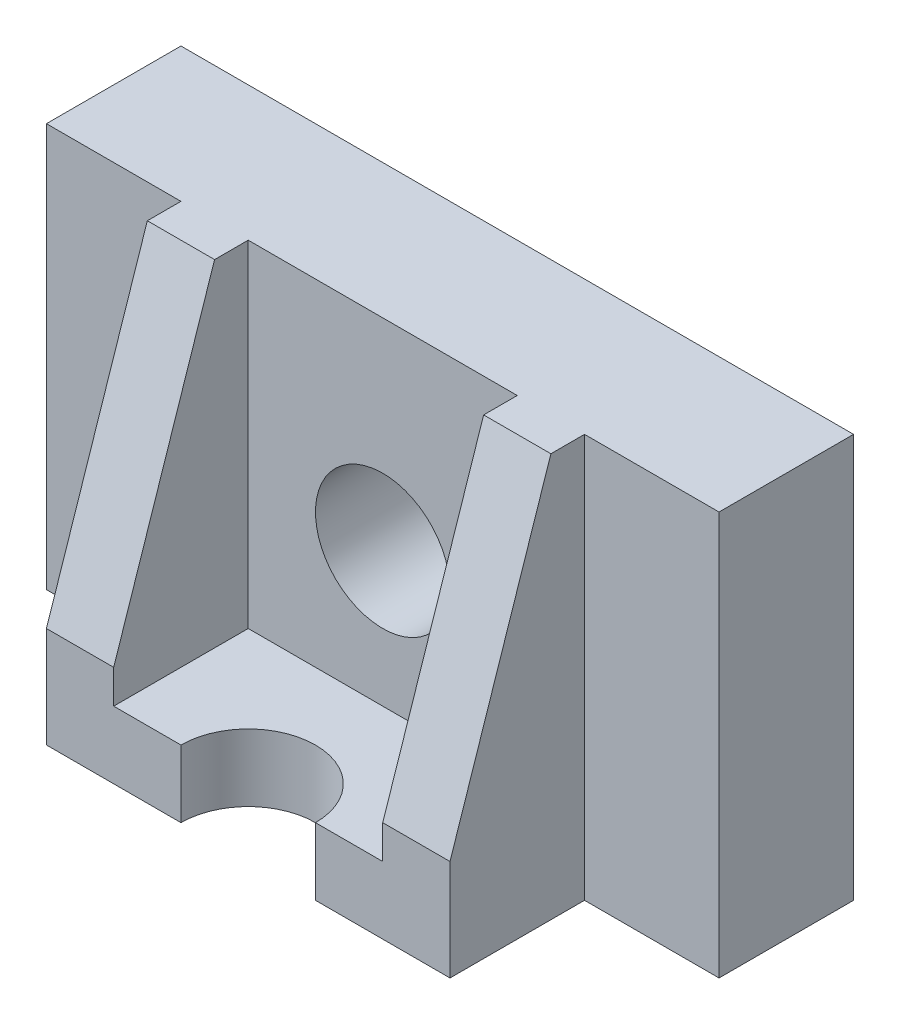
ISO-10303-21;
HEADER;
FILE_DESCRIPTION(('STEP AP214'),'2;1');
FILE_NAME('part.step','',(''),(''),'','','');
FILE_SCHEMA(('AUTOMOTIVE_DESIGN { 1 0 10303 214 1 1 1 1 }'));
ENDSEC;
DATA;
#1=APPLICATION_CONTEXT('core data for automotive mechanical design processes');
#2=APPLICATION_PROTOCOL_DEFINITION('international standard','automotive_design',2000,#1);
#3=PRODUCT_CONTEXT('',#1,'mechanical');
#4=PRODUCT('Part','Part','',(#3));
#5=PRODUCT_RELATED_PRODUCT_CATEGORY('part','',(#4));
#6=PRODUCT_DEFINITION_FORMATION('','',#4);
#7=PRODUCT_DEFINITION_CONTEXT('part definition',#1,'design');
#8=PRODUCT_DEFINITION('design','',#6,#7);
#9=PRODUCT_DEFINITION_SHAPE('','',#8);
#10=(LENGTH_UNIT() NAMED_UNIT(*) SI_UNIT(.MILLI.,.METRE.));
#11=(NAMED_UNIT(*) PLANE_ANGLE_UNIT() SI_UNIT($,.RADIAN.));
#12=(NAMED_UNIT(*) SI_UNIT($,.STERADIAN.) SOLID_ANGLE_UNIT());
#13=UNCERTAINTY_MEASURE_WITH_UNIT(LENGTH_MEASURE(1.E-05),#10,'distance_accuracy_value','');
#14=(GEOMETRIC_REPRESENTATION_CONTEXT(3) GLOBAL_UNCERTAINTY_ASSIGNED_CONTEXT((#13)) GLOBAL_UNIT_ASSIGNED_CONTEXT((#10,
#11,#12)) REPRESENTATION_CONTEXT('',''));
#15=CARTESIAN_POINT('',(0.,0.,0.));
#16=DIRECTION('',(0.,0.,1.));
#17=DIRECTION('',(1.,0.,0.));
#18=AXIS2_PLACEMENT_3D('',#15,#16,#17);
#19=CARTESIAN_POINT('',(0.,0.,20.));
#20=DIRECTION('',(0.,0.,1.));
#21=DIRECTION('',(1.,0.,0.));
#22=AXIS2_PLACEMENT_3D('',#19,#20,#21);
#23=PLANE('',#22);
#24=CARTESIAN_POINT('',(50.,30.,20.));
#25=DIRECTION('',(0.,0.,1.));
#26=DIRECTION('',(1.,0.,0.));
#27=AXIS2_PLACEMENT_3D('',#24,#25,#26);
#28=CIRCLE('',#27,10.);
#29=CARTESIAN_POINT('',(60.,30.,20.));
#30=VERTEX_POINT('',#29);
#31=EDGE_CURVE('E217',#30,#30,#28,.T.);
#32=ORIENTED_EDGE('',*,*,#31,.F.);
#33=EDGE_LOOP('',(#32));
#34=FACE_BOUND('',#33,.T.);
#35=DIRECTION('',(-1.,0.,0.));
#36=VECTOR('',#35,1.);
#37=CARTESIAN_POINT('',(100.,60.,20.));
#38=LINE('',#37,#36);
#39=CARTESIAN_POINT('',(70.,60.,20.));
#40=VERTEX_POINT('',#39);
#41=CARTESIAN_POINT('',(30.,60.,20.));
#42=VERTEX_POINT('',#41);
#43=EDGE_CURVE('E245',#40,#42,#38,.T.);
#44=ORIENTED_EDGE('',*,*,#43,.T.);
#45=DIRECTION('',(0.,-1.,0.));
#46=VECTOR('',#45,1.);
#47=CARTESIAN_POINT('',(30.,60.,20.));
#48=LINE('',#47,#46);
#49=CARTESIAN_POINT('',(30.,10.,20.));
#50=VERTEX_POINT('',#49);
#51=EDGE_CURVE('E274',#42,#50,#48,.T.);
#52=ORIENTED_EDGE('',*,*,#51,.T.);
#53=DIRECTION('',(1.,0.,0.));
#54=VECTOR('',#53,1.);
#55=CARTESIAN_POINT('',(20.,10.,20.));
#56=LINE('',#55,#54);
#57=CARTESIAN_POINT('',(70.,10.,20.));
#58=VERTEX_POINT('',#57);
#59=EDGE_CURVE('E186',#50,#58,#56,.T.);
#60=ORIENTED_EDGE('',*,*,#59,.T.);
#61=DIRECTION('',(0.,1.,0.));
#62=VECTOR('',#61,1.);
#63=CARTESIAN_POINT('',(70.,60.,20.));
#64=LINE('',#63,#62);
#65=EDGE_CURVE('E277',#58,#40,#64,.T.);
#66=ORIENTED_EDGE('',*,*,#65,.T.);
#67=EDGE_LOOP('',(#44,#52,#60,#66));
#68=FACE_BOUND('',#67,.T.);
#69=ADVANCED_FACE('F44',(#34,#68),#23,.T.);
#70=CARTESIAN_POINT('',(50.,10.,40.));
#71=DIRECTION('',(0.,-1.,0.));
#72=DIRECTION('',(0.,0.,-1.));
#73=AXIS2_PLACEMENT_3D('',#70,#71,#72);
#74=PLANE('',#73);
#75=DIRECTION('',(0.,0.,1.));
#76=VECTOR('',#75,1.);
#77=CARTESIAN_POINT('',(30.,10.,20.));
#78=LINE('',#77,#76);
#79=CARTESIAN_POINT('',(30.,10.,40.));
#80=VERTEX_POINT('',#79);
#81=EDGE_CURVE('E175',#50,#80,#78,.T.);
#82=ORIENTED_EDGE('',*,*,#81,.T.);
#83=DIRECTION('',(-1.,0.,0.));
#84=VECTOR('',#83,1.);
#85=CARTESIAN_POINT('',(20.,10.,40.));
#86=LINE('',#85,#84);
#87=CARTESIAN_POINT('',(40.,10.,40.));
#88=VERTEX_POINT('',#87);
#89=EDGE_CURVE('E187',#88,#80,#86,.T.);
#90=ORIENTED_EDGE('',*,*,#89,.F.);
#91=CARTESIAN_POINT('',(50.,10.,40.));
#92=DIRECTION('',(0.,1.,0.));
#93=DIRECTION('',(0.,0.,-1.));
#94=AXIS2_PLACEMENT_3D('',#91,#92,#93);
#95=CIRCLE('',#94,10.);
#96=CARTESIAN_POINT('',(60.,10.,40.));
#97=VERTEX_POINT('',#96);
#98=EDGE_CURVE('E196',#97,#88,#95,.T.);
#99=ORIENTED_EDGE('',*,*,#98,.F.);
#100=DIRECTION('',(-1.,0.,0.));
#101=VECTOR('',#100,1.);
#102=CARTESIAN_POINT('',(80.,10.,40.));
#103=LINE('',#102,#101);
#104=CARTESIAN_POINT('',(70.,10.,40.));
#105=VERTEX_POINT('',#104);
#106=EDGE_CURVE('E199',#105,#97,#103,.T.);
#107=ORIENTED_EDGE('',*,*,#106,.F.);
#108=DIRECTION('',(0.,0.,-1.));
#109=VECTOR('',#108,1.);
#110=CARTESIAN_POINT('',(70.,10.,20.));
#111=LINE('',#110,#109);
#112=EDGE_CURVE('E292',#105,#58,#111,.T.);
#113=ORIENTED_EDGE('',*,*,#112,.T.);
#114=ORIENTED_EDGE('',*,*,#59,.F.);
#115=EDGE_LOOP('',(#82,#90,#99,#107,#113,#114));
#116=FACE_BOUND('',#115,.T.);
#117=ADVANCED_FACE('F183',(#116),#74,.F.);
#118=CARTESIAN_POINT('',(100.,60.,20.));
#119=VERTEX_POINT('',#118);
#120=CARTESIAN_POINT('',(80.,60.,20.));
#121=VERTEX_POINT('',#120);
#122=EDGE_CURVE('E238',#119,#121,#38,.T.);
#123=ORIENTED_EDGE('',*,*,#122,.T.);
#124=DIRECTION('',(0.,-1.,0.));
#125=VECTOR('',#124,1.);
#126=CARTESIAN_POINT('',(80.,10.,20.));
#127=LINE('',#126,#125);
#128=CARTESIAN_POINT('',(80.,0.,20.));
#129=VERTEX_POINT('',#128);
#130=EDGE_CURVE('E193',#121,#129,#127,.T.);
#131=ORIENTED_EDGE('',*,*,#130,.T.);
#132=DIRECTION('',(1.,0.,0.));
#133=VECTOR('',#132,1.);
#134=CARTESIAN_POINT('',(0.,0.,20.));
#135=LINE('',#134,#133);
#136=CARTESIAN_POINT('',(100.,0.,20.));
#137=VERTEX_POINT('',#136);
#138=EDGE_CURVE('E234',#129,#137,#135,.T.);
#139=ORIENTED_EDGE('',*,*,#138,.T.);
#140=DIRECTION('',(0.,1.,0.));
#141=VECTOR('',#140,1.);
#142=CARTESIAN_POINT('',(100.,0.,20.));
#143=LINE('',#142,#141);
#144=EDGE_CURVE('E236',#137,#119,#143,.T.);
#145=ORIENTED_EDGE('',*,*,#144,.T.);
#146=EDGE_LOOP('',(#123,#131,#139,#145));
#147=FACE_BOUND('',#146,.T.);
#148=ADVANCED_FACE('F327',(#147),#23,.T.);
#149=CARTESIAN_POINT('',(0.,60.,20.));
#150=DIRECTION('',(1.,0.,0.));
#151=DIRECTION('',(0.,0.,-1.));
#152=AXIS2_PLACEMENT_3D('',#149,#150,#151);
#153=PLANE('',#152);
#154=DIRECTION('',(0.,-1.,0.));
#155=VECTOR('',#154,1.);
#156=CARTESIAN_POINT('',(0.,60.,0.));
#157=LINE('',#156,#155);
#158=CARTESIAN_POINT('',(0.,60.,0.));
#159=VERTEX_POINT('',#158);
#160=CARTESIAN_POINT('',(0.,0.,0.));
#161=VERTEX_POINT('',#160);
#162=EDGE_CURVE('E230',#159,#161,#157,.T.);
#163=ORIENTED_EDGE('',*,*,#162,.T.);
#164=DIRECTION('',(0.,0.,-1.));
#165=VECTOR('',#164,1.);
#166=CARTESIAN_POINT('',(0.,0.,20.));
#167=LINE('',#166,#165);
#168=CARTESIAN_POINT('',(0.,0.,20.));
#169=VERTEX_POINT('',#168);
#170=EDGE_CURVE('E11',#169,#161,#167,.T.);
#171=ORIENTED_EDGE('',*,*,#170,.F.);
#172=DIRECTION('',(0.,-1.,0.));
#173=VECTOR('',#172,1.);
#174=CARTESIAN_POINT('',(0.,60.,20.));
#175=LINE('',#174,#173);
#176=CARTESIAN_POINT('',(0.,60.,20.));
#177=VERTEX_POINT('',#176);
#178=EDGE_CURVE('E235',#177,#169,#175,.T.);
#179=ORIENTED_EDGE('',*,*,#178,.F.);
#180=DIRECTION('',(0.,0.,-1.));
#181=VECTOR('',#180,1.);
#182=CARTESIAN_POINT('',(0.,60.,20.));
#183=LINE('',#182,#181);
#184=EDGE_CURVE('E241',#177,#159,#183,.T.);
#185=ORIENTED_EDGE('',*,*,#184,.T.);
#186=EDGE_LOOP('',(#163,#171,#179,#185));
#187=FACE_BOUND('',#186,.T.);
#188=ADVANCED_FACE('F50',(#187),#153,.F.);
#189=CARTESIAN_POINT('',(0.,0.,20.));
#190=DIRECTION('',(0.,1.,0.));
#191=DIRECTION('',(0.,0.,1.));
#192=AXIS2_PLACEMENT_3D('',#189,#190,#191);
#193=PLANE('',#192);
#194=DIRECTION('',(1.,0.,0.));
#195=VECTOR('',#194,1.);
#196=CARTESIAN_POINT('',(0.,0.,0.));
#197=LINE('',#196,#195);
#198=CARTESIAN_POINT('',(100.,0.,0.));
#199=VERTEX_POINT('',#198);
#200=EDGE_CURVE('E244',#161,#199,#197,.T.);
#201=ORIENTED_EDGE('',*,*,#200,.T.);
#202=DIRECTION('',(0.,0.,-1.));
#203=VECTOR('',#202,1.);
#204=CARTESIAN_POINT('',(100.,0.,20.));
#205=LINE('',#204,#203);
#206=EDGE_CURVE('E52',#137,#199,#205,.T.);
#207=ORIENTED_EDGE('',*,*,#206,.F.);
#208=ORIENTED_EDGE('',*,*,#138,.F.);
#209=DIRECTION('',(0.,0.,1.));
#210=VECTOR('',#209,1.);
#211=CARTESIAN_POINT('',(80.,0.,20.));
#212=LINE('',#211,#210);
#213=CARTESIAN_POINT('',(80.,0.,40.));
#214=VERTEX_POINT('',#213);
#215=EDGE_CURVE('E58',#129,#214,#212,.T.);
#216=ORIENTED_EDGE('',*,*,#215,.T.);
#217=DIRECTION('',(-1.,0.,0.));
#218=VECTOR('',#217,1.);
#219=CARTESIAN_POINT('',(80.,0.,40.));
#220=LINE('',#219,#218);
#221=CARTESIAN_POINT('',(60.,0.,40.));
#222=VERTEX_POINT('',#221);
#223=EDGE_CURVE('E205',#214,#222,#220,.T.);
#224=ORIENTED_EDGE('',*,*,#223,.T.);
#225=CARTESIAN_POINT('',(50.,0.,40.));
#226=DIRECTION('',(0.,1.,0.));
#227=DIRECTION('',(0.,0.,-1.));
#228=AXIS2_PLACEMENT_3D('',#225,#226,#227);
#229=CIRCLE('',#228,10.);
#230=CARTESIAN_POINT('',(40.,0.,40.));
#231=VERTEX_POINT('',#230);
#232=EDGE_CURVE('E209',#222,#231,#229,.T.);
#233=ORIENTED_EDGE('',*,*,#232,.T.);
#234=DIRECTION('',(-1.,0.,0.));
#235=VECTOR('',#234,1.);
#236=CARTESIAN_POINT('',(20.,0.,40.));
#237=LINE('',#236,#235);
#238=CARTESIAN_POINT('',(20.,0.,40.));
#239=VERTEX_POINT('',#238);
#240=EDGE_CURVE('E215',#231,#239,#237,.T.);
#241=ORIENTED_EDGE('',*,*,#240,.T.);
#242=DIRECTION('',(0.,0.,-1.));
#243=VECTOR('',#242,1.);
#244=CARTESIAN_POINT('',(20.,0.,20.));
#245=LINE('',#244,#243);
#246=CARTESIAN_POINT('',(20.,0.,20.));
#247=VERTEX_POINT('',#246);
#248=EDGE_CURVE('E213',#239,#247,#245,.T.);
#249=ORIENTED_EDGE('',*,*,#248,.T.);
#250=EDGE_CURVE('E96',#169,#247,#135,.T.);
#251=ORIENTED_EDGE('',*,*,#250,.F.);
#252=ORIENTED_EDGE('',*,*,#170,.T.);
#253=EDGE_LOOP('',(#201,#207,#208,#216,#224,#233,#241,#249,#251,#252));
#254=FACE_BOUND('',#253,.T.);
#255=ADVANCED_FACE('F318',(#254),#193,.F.);
#256=CARTESIAN_POINT('',(100.,0.,20.));
#257=DIRECTION('',(-1.,0.,0.));
#258=DIRECTION('',(0.,0.,1.));
#259=AXIS2_PLACEMENT_3D('',#256,#257,#258);
#260=PLANE('',#259);
#261=DIRECTION('',(0.,1.,0.));
#262=VECTOR('',#261,1.);
#263=CARTESIAN_POINT('',(100.,0.,0.));
#264=LINE('',#263,#262);
#265=CARTESIAN_POINT('',(100.,60.,0.));
#266=VERTEX_POINT('',#265);
#267=EDGE_CURVE('E250',#199,#266,#264,.T.);
#268=ORIENTED_EDGE('',*,*,#267,.T.);
#269=DIRECTION('',(0.,0.,-1.));
#270=VECTOR('',#269,1.);
#271=CARTESIAN_POINT('',(100.,60.,20.));
#272=LINE('',#271,#270);
#273=EDGE_CURVE('E252',#119,#266,#272,.T.);
#274=ORIENTED_EDGE('',*,*,#273,.F.);
#275=ORIENTED_EDGE('',*,*,#144,.F.);
#276=ORIENTED_EDGE('',*,*,#206,.T.);
#277=EDGE_LOOP('',(#268,#274,#275,#276));
#278=FACE_BOUND('',#277,.T.);
#279=ADVANCED_FACE('F260',(#278),#260,.F.);
#280=CARTESIAN_POINT('',(100.,60.,20.));
#281=DIRECTION('',(0.,-1.,0.));
#282=DIRECTION('',(0.,0.,-1.));
#283=AXIS2_PLACEMENT_3D('',#280,#281,#282);
#284=PLANE('',#283);
#285=DIRECTION('',(-1.,0.,0.));
#286=VECTOR('',#285,1.);
#287=CARTESIAN_POINT('',(100.,60.,0.));
#288=LINE('',#287,#286);
#289=EDGE_CURVE('E91',#266,#159,#288,.T.);
#290=ORIENTED_EDGE('',*,*,#289,.T.);
#291=ORIENTED_EDGE('',*,*,#184,.F.);
#292=CARTESIAN_POINT('',(20.,60.,20.));
#293=VERTEX_POINT('',#292);
#294=EDGE_CURVE('E67',#293,#177,#38,.T.);
#295=ORIENTED_EDGE('',*,*,#294,.F.);
#296=DIRECTION('',(0.,0.,-1.));
#297=VECTOR('',#296,1.);
#298=CARTESIAN_POINT('',(20.,60.,25.));
#299=LINE('',#298,#297);
#300=CARTESIAN_POINT('',(20.,60.,25.));
#301=VERTEX_POINT('',#300);
#302=EDGE_CURVE('E188',#301,#293,#299,.T.);
#303=ORIENTED_EDGE('',*,*,#302,.F.);
#304=DIRECTION('',(-1.,0.,0.));
#305=VECTOR('',#304,1.);
#306=CARTESIAN_POINT('',(30.,60.,25.));
#307=LINE('',#306,#305);
#308=CARTESIAN_POINT('',(30.,60.,25.));
#309=VERTEX_POINT('',#308);
#310=EDGE_CURVE('E278',#309,#301,#307,.T.);
#311=ORIENTED_EDGE('',*,*,#310,.F.);
#312=DIRECTION('',(0.,0.,-1.));
#313=VECTOR('',#312,1.);
#314=CARTESIAN_POINT('',(30.,60.,25.));
#315=LINE('',#314,#313);
#316=EDGE_CURVE('E276',#309,#42,#315,.T.);
#317=ORIENTED_EDGE('',*,*,#316,.T.);
#318=ORIENTED_EDGE('',*,*,#43,.F.);
#319=DIRECTION('',(0.,0.,1.));
#320=VECTOR('',#319,1.);
#321=CARTESIAN_POINT('',(70.,60.,20.));
#322=LINE('',#321,#320);
#323=CARTESIAN_POINT('',(70.,60.,25.));
#324=VERTEX_POINT('',#323);
#325=EDGE_CURVE('E279',#40,#324,#322,.T.);
#326=ORIENTED_EDGE('',*,*,#325,.T.);
#327=DIRECTION('',(1.,0.,0.));
#328=VECTOR('',#327,1.);
#329=CARTESIAN_POINT('',(70.,60.,25.));
#330=LINE('',#329,#328);
#331=CARTESIAN_POINT('',(80.,60.,25.));
#332=VERTEX_POINT('',#331);
#333=EDGE_CURVE('E303',#324,#332,#330,.T.);
#334=ORIENTED_EDGE('',*,*,#333,.T.);
#335=DIRECTION('',(0.,0.,1.));
#336=VECTOR('',#335,1.);
#337=CARTESIAN_POINT('',(80.,60.,20.));
#338=LINE('',#337,#336);
#339=EDGE_CURVE('E290',#121,#332,#338,.T.);
#340=ORIENTED_EDGE('',*,*,#339,.F.);
#341=ORIENTED_EDGE('',*,*,#122,.F.);
#342=ORIENTED_EDGE('',*,*,#273,.T.);
#343=EDGE_LOOP('',(#290,#291,#295,#303,#311,#317,#318,#326,#334,#340,#341,#342));
#344=FACE_BOUND('',#343,.T.);
#345=ADVANCED_FACE('F266',(#344),#284,.F.);
#346=DIRECTION('',(0.,-1.,0.));
#347=VECTOR('',#346,1.);
#348=CARTESIAN_POINT('',(20.,10.,20.));
#349=LINE('',#348,#347);
#350=EDGE_CURVE('E220',#293,#247,#349,.T.);
#351=ORIENTED_EDGE('',*,*,#350,.F.);
#352=ORIENTED_EDGE('',*,*,#294,.T.);
#353=ORIENTED_EDGE('',*,*,#178,.T.);
#354=ORIENTED_EDGE('',*,*,#250,.T.);
#355=EDGE_LOOP('',(#351,#352,#353,#354));
#356=FACE_BOUND('',#355,.T.);
#357=ADVANCED_FACE('F332',(#356),#23,.T.);
#358=CARTESIAN_POINT('',(0.,0.,0.));
#359=DIRECTION('',(0.,0.,1.));
#360=DIRECTION('',(1.,0.,0.));
#361=AXIS2_PLACEMENT_3D('',#358,#359,#360);
#362=PLANE('',#361);
#363=CARTESIAN_POINT('',(50.,30.,0.));
#364=DIRECTION('',(0.,0.,1.));
#365=DIRECTION('',(1.,0.,0.));
#366=AXIS2_PLACEMENT_3D('',#363,#364,#365);
#367=CIRCLE('',#366,10.);
#368=CARTESIAN_POINT('',(60.,30.,0.));
#369=VERTEX_POINT('',#368);
#370=EDGE_CURVE('E228',#369,#369,#367,.T.);
#371=ORIENTED_EDGE('',*,*,#370,.T.);
#372=EDGE_LOOP('',(#371));
#373=FACE_BOUND('',#372,.T.);
#374=ORIENTED_EDGE('',*,*,#162,.F.);
#375=ORIENTED_EDGE('',*,*,#289,.F.);
#376=ORIENTED_EDGE('',*,*,#267,.F.);
#377=ORIENTED_EDGE('',*,*,#200,.F.);
#378=EDGE_LOOP('',(#374,#375,#376,#377));
#379=FACE_BOUND('',#378,.T.);
#380=ADVANCED_FACE('F265',(#373,#379),#362,.F.);
#381=CARTESIAN_POINT('',(50.,30.,0.));
#382=DIRECTION('',(0.,0.,1.));
#383=DIRECTION('',(1.,0.,0.));
#384=AXIS2_PLACEMENT_3D('',#381,#382,#383);
#385=CYLINDRICAL_SURFACE('',#384,10.);
#386=ORIENTED_EDGE('',*,*,#370,.F.);
#387=EDGE_LOOP('',(#386));
#388=FACE_BOUND('',#387,.T.);
#389=ORIENTED_EDGE('',*,*,#31,.T.);
#390=EDGE_LOOP('',(#389));
#391=FACE_BOUND('',#390,.T.);
#392=ADVANCED_FACE('F350',(#388,#391),#385,.F.);
#393=CARTESIAN_POINT('',(20.,10.,20.));
#394=DIRECTION('',(-1.,0.,0.));
#395=DIRECTION('',(0.,0.,1.));
#396=AXIS2_PLACEMENT_3D('',#393,#394,#395);
#397=PLANE('',#396);
#398=ORIENTED_EDGE('',*,*,#248,.F.);
#399=DIRECTION('',(0.,-1.,0.));
#400=VECTOR('',#399,1.);
#401=CARTESIAN_POINT('',(20.,10.,40.));
#402=LINE('',#401,#400);
#403=CARTESIAN_POINT('',(20.,15.,40.));
#404=VERTEX_POINT('',#403);
#405=EDGE_CURVE('E219',#404,#239,#402,.T.);
#406=ORIENTED_EDGE('',*,*,#405,.F.);
#407=DIRECTION('',(0.,0.948683298050514,-0.316227766016838));
#408=VECTOR('',#407,1.);
#409=CARTESIAN_POINT('',(20.,15.,40.));
#410=LINE('',#409,#408);
#411=EDGE_CURVE('E287',#404,#301,#410,.T.);
#412=ORIENTED_EDGE('',*,*,#411,.T.);
#413=ORIENTED_EDGE('',*,*,#302,.T.);
#414=ORIENTED_EDGE('',*,*,#350,.T.);
#415=EDGE_LOOP('',(#398,#406,#412,#413,#414));
#416=FACE_BOUND('',#415,.T.);
#417=ADVANCED_FACE('F347',(#416),#397,.T.);
#418=CARTESIAN_POINT('',(20.,10.,40.));
#419=DIRECTION('',(0.,0.,1.));
#420=DIRECTION('',(1.,0.,0.));
#421=AXIS2_PLACEMENT_3D('',#418,#419,#420);
#422=PLANE('',#421);
#423=ORIENTED_EDGE('',*,*,#240,.F.);
#424=DIRECTION('',(0.,-1.,0.));
#425=VECTOR('',#424,1.);
#426=CARTESIAN_POINT('',(40.,10.,40.));
#427=LINE('',#426,#425);
#428=EDGE_CURVE('E191',#88,#231,#427,.T.);
#429=ORIENTED_EDGE('',*,*,#428,.F.);
#430=ORIENTED_EDGE('',*,*,#89,.T.);
#431=DIRECTION('',(0.,1.,0.));
#432=VECTOR('',#431,1.);
#433=CARTESIAN_POINT('',(30.,10.,40.));
#434=LINE('',#433,#432);
#435=CARTESIAN_POINT('',(30.,15.,40.));
#436=VERTEX_POINT('',#435);
#437=EDGE_CURVE('E166',#80,#436,#434,.T.);
#438=ORIENTED_EDGE('',*,*,#437,.T.);
#439=DIRECTION('',(-1.,0.,0.));
#440=VECTOR('',#439,1.);
#441=CARTESIAN_POINT('',(30.,15.,40.));
#442=LINE('',#441,#440);
#443=EDGE_CURVE('E285',#436,#404,#442,.T.);
#444=ORIENTED_EDGE('',*,*,#443,.T.);
#445=ORIENTED_EDGE('',*,*,#405,.T.);
#446=EDGE_LOOP('',(#423,#429,#430,#438,#444,#445));
#447=FACE_BOUND('',#446,.T.);
#448=ADVANCED_FACE('F194',(#447),#422,.T.);
#449=CARTESIAN_POINT('',(50.,10.,40.));
#450=DIRECTION('',(0.,-1.,0.));
#451=DIRECTION('',(0.,0.,-1.));
#452=AXIS2_PLACEMENT_3D('',#449,#450,#451);
#453=CYLINDRICAL_SURFACE('',#452,10.);
#454=ORIENTED_EDGE('',*,*,#232,.F.);
#455=DIRECTION('',(0.,-1.,0.));
#456=VECTOR('',#455,1.);
#457=CARTESIAN_POINT('',(60.,10.,40.));
#458=LINE('',#457,#456);
#459=EDGE_CURVE('E224',#97,#222,#458,.T.);
#460=ORIENTED_EDGE('',*,*,#459,.F.);
#461=ORIENTED_EDGE('',*,*,#98,.T.);
#462=ORIENTED_EDGE('',*,*,#428,.T.);
#463=EDGE_LOOP('',(#454,#460,#461,#462));
#464=FACE_BOUND('',#463,.T.);
#465=ADVANCED_FACE('F316',(#464),#453,.F.);
#466=CARTESIAN_POINT('',(80.,10.,40.));
#467=DIRECTION('',(0.,0.,1.));
#468=DIRECTION('',(1.,0.,0.));
#469=AXIS2_PLACEMENT_3D('',#466,#467,#468);
#470=PLANE('',#469);
#471=ORIENTED_EDGE('',*,*,#223,.F.);
#472=DIRECTION('',(0.,-1.,0.));
#473=VECTOR('',#472,1.);
#474=CARTESIAN_POINT('',(80.,10.,40.));
#475=LINE('',#474,#473);
#476=CARTESIAN_POINT('',(80.,15.,40.));
#477=VERTEX_POINT('',#476);
#478=EDGE_CURVE('E198',#477,#214,#475,.T.);
#479=ORIENTED_EDGE('',*,*,#478,.F.);
#480=DIRECTION('',(1.,0.,0.));
#481=VECTOR('',#480,1.);
#482=CARTESIAN_POINT('',(70.,15.,40.));
#483=LINE('',#482,#481);
#484=CARTESIAN_POINT('',(70.,15.,40.));
#485=VERTEX_POINT('',#484);
#486=EDGE_CURVE('E207',#485,#477,#483,.T.);
#487=ORIENTED_EDGE('',*,*,#486,.F.);
#488=DIRECTION('',(0.,-1.,0.));
#489=VECTOR('',#488,1.);
#490=CARTESIAN_POINT('',(70.,10.,40.));
#491=LINE('',#490,#489);
#492=EDGE_CURVE('E297',#485,#105,#491,.T.);
#493=ORIENTED_EDGE('',*,*,#492,.T.);
#494=ORIENTED_EDGE('',*,*,#106,.T.);
#495=ORIENTED_EDGE('',*,*,#459,.T.);
#496=EDGE_LOOP('',(#471,#479,#487,#493,#494,#495));
#497=FACE_BOUND('',#496,.T.);
#498=ADVANCED_FACE('F314',(#497),#470,.T.);
#499=CARTESIAN_POINT('',(80.,10.,20.));
#500=DIRECTION('',(1.,0.,0.));
#501=DIRECTION('',(0.,0.,-1.));
#502=AXIS2_PLACEMENT_3D('',#499,#500,#501);
#503=PLANE('',#502);
#504=ORIENTED_EDGE('',*,*,#215,.F.);
#505=ORIENTED_EDGE('',*,*,#130,.F.);
#506=ORIENTED_EDGE('',*,*,#339,.T.);
#507=DIRECTION('',(0.,-0.948683298050514,0.316227766016838));
#508=VECTOR('',#507,1.);
#509=CARTESIAN_POINT('',(80.,60.,25.));
#510=LINE('',#509,#508);
#511=EDGE_CURVE('E295',#332,#477,#510,.T.);
#512=ORIENTED_EDGE('',*,*,#511,.T.);
#513=ORIENTED_EDGE('',*,*,#478,.T.);
#514=EDGE_LOOP('',(#504,#505,#506,#512,#513));
#515=FACE_BOUND('',#514,.T.);
#516=ADVANCED_FACE('F323',(#515),#503,.T.);
#517=CARTESIAN_POINT('',(70.,60.,25.));
#518=DIRECTION('',(0.,0.316227766016838,0.948683298050514));
#519=DIRECTION('',(0.,-0.948683298050514,0.316227766016838));
#520=AXIS2_PLACEMENT_3D('',#517,#518,#519);
#521=PLANE('',#520);
#522=ORIENTED_EDGE('',*,*,#511,.F.);
#523=ORIENTED_EDGE('',*,*,#333,.F.);
#524=DIRECTION('',(0.,-0.948683298050514,0.316227766016838));
#525=VECTOR('',#524,1.);
#526=CARTESIAN_POINT('',(70.,60.,25.));
#527=LINE('',#526,#525);
#528=EDGE_CURVE('E300',#324,#485,#527,.T.);
#529=ORIENTED_EDGE('',*,*,#528,.T.);
#530=ORIENTED_EDGE('',*,*,#486,.T.);
#531=EDGE_LOOP('',(#522,#523,#529,#530));
#532=FACE_BOUND('',#531,.T.);
#533=ADVANCED_FACE('F324',(#532),#521,.T.);
#534=CARTESIAN_POINT('',(70.,0.,0.));
#535=DIRECTION('',(-1.,0.,0.));
#536=DIRECTION('',(0.,0.,1.));
#537=AXIS2_PLACEMENT_3D('',#534,#535,#536);
#538=PLANE('',#537);
#539=ORIENTED_EDGE('',*,*,#112,.F.);
#540=ORIENTED_EDGE('',*,*,#492,.F.);
#541=ORIENTED_EDGE('',*,*,#528,.F.);
#542=ORIENTED_EDGE('',*,*,#325,.F.);
#543=ORIENTED_EDGE('',*,*,#65,.F.);
#544=EDGE_LOOP('',(#539,#540,#541,#542,#543));
#545=FACE_BOUND('',#544,.T.);
#546=ADVANCED_FACE('F375',(#545),#538,.T.);
#547=CARTESIAN_POINT('',(30.,15.,40.));
#548=DIRECTION('',(0.,0.316227766016838,0.948683298050514));
#549=DIRECTION('',(0.,-0.948683298050514,0.316227766016838));
#550=AXIS2_PLACEMENT_3D('',#547,#548,#549);
#551=PLANE('',#550);
#552=ORIENTED_EDGE('',*,*,#411,.F.);
#553=ORIENTED_EDGE('',*,*,#443,.F.);
#554=DIRECTION('',(0.,0.948683298050514,-0.316227766016838));
#555=VECTOR('',#554,1.);
#556=CARTESIAN_POINT('',(30.,15.,40.));
#557=LINE('',#556,#555);
#558=EDGE_CURVE('E176',#436,#309,#557,.T.);
#559=ORIENTED_EDGE('',*,*,#558,.T.);
#560=ORIENTED_EDGE('',*,*,#310,.T.);
#561=EDGE_LOOP('',(#552,#553,#559,#560));
#562=FACE_BOUND('',#561,.T.);
#563=ADVANCED_FACE('F374',(#562),#551,.T.);
#564=CARTESIAN_POINT('',(30.,0.,0.));
#565=DIRECTION('',(-1.,0.,0.));
#566=DIRECTION('',(0.,0.,1.));
#567=AXIS2_PLACEMENT_3D('',#564,#565,#566);
#568=PLANE('',#567);
#569=ORIENTED_EDGE('',*,*,#81,.F.);
#570=ORIENTED_EDGE('',*,*,#51,.F.);
#571=ORIENTED_EDGE('',*,*,#316,.F.);
#572=ORIENTED_EDGE('',*,*,#558,.F.);
#573=ORIENTED_EDGE('',*,*,#437,.F.);
#574=EDGE_LOOP('',(#569,#570,#571,#572,#573));
#575=FACE_BOUND('',#574,.T.);
#576=ADVANCED_FACE('F167',(#575),#568,.F.);
#577=CLOSED_SHELL('',(#69,#117,#148,#188,#255,#279,#345,#357,#380,#392,#417,#448,#465,#498,#516,
#533,#546,#563,#576));
#578=MANIFOLD_SOLID_BREP('B2',#577);
#579=ADVANCED_BREP_SHAPE_REPRESENTATION('',(#18,#578),#14);
#580=SHAPE_DEFINITION_REPRESENTATION(#9,#579);
ENDSEC;
END-ISO-10303-21;
